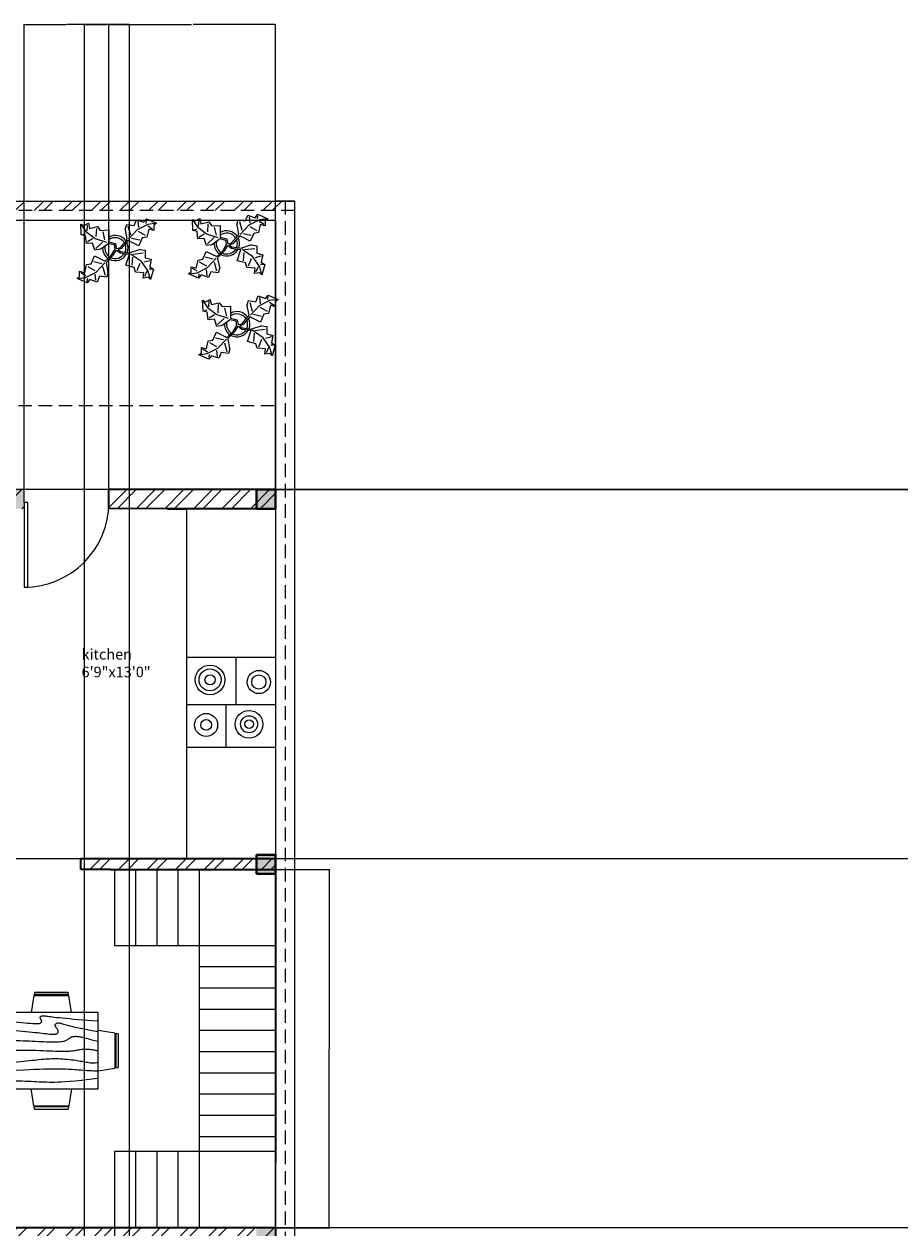
# Model space of a CAD drawing. Units: inches. Extents: x 19613 to 21413, y 12082 to 13202.
# Tile 6 of 9: x 20100 to 20513, y 12634 to 13202. Entities that reach past the tile are written whole.
import ezdxf

# ---------------------------------------------------------------- set-up
doc = ezdxf.new("R2010")
doc.units = ezdxf.units.IN
doc.linetypes.add('HIDDEN', pattern=[9.525, 6.35, -3.175])
for name, color, linetype, lineweight in [('A-ANNO-DIMS', 2, 'Continuous', 18), ('A-AREA-IDEN', 7, 'Continuous', 18), ('A-COLS', 7, 'Continuous', 40), ('A-COLS-PATT', 6, 'Continuous', 13), ('A-DOOR', 3, 'Continuous', 18), ('A-EQPM', 8, 'Continuous', 18), ('A-FLOR-CASE', 9, 'Continuous', 18), ('A-FLOR-HIDN', 8, 'HIDDEN', 13), ('A-FLOR-STRS', 7, 'Continuous', 18), ('A-FURN', 8, 'Continuous', 18), ('A-WALL', 7, 'Continuous', 35), ('A-WALL-PATT', 252, 'Continuous', 13), ('C-PROP', 7, 'Continuous', 25), ('C-PROP-HIDN', 8, 'HIDDEN', 13), ('L-PLNT', 116, 'Continuous', 18)]:
    doc.layers.add(name, color=color, linetype=linetype, lineweight=lineweight)
doc.styles.get("Standard").update_dxf_attribs({"font": 'arial.ttf'})
doc.dimstyles.get("Standard").update_dxf_attribs({"dimtxt": 0.18, "dimasz": 0.18, "dimexe": 0.18, "dimexo": 0.0625, "dimgap": 0.09, "dimtad": 0, "dimtih": 1, "dimtoh": 1, "dimdec": 4, "dimzin": 0, "dimdsep": 46, "dimtxsty": 'Standard', "dimcen": 0.09, "dimadec": 0, "dimazin": 0, "dimtfac": 1, "dimtdec": 4, "dimtofl": 0, "dimtmove": 0, "dimatfit": 3, "dimfxl": 1, "dimtolj": 1, "dimtzin": 0, "dimarcsym": 0})

# ---------------------------------------------------------------- blocks, each defined once
blk = doc.blocks.new('*U2')
for p, q in [((0, 0), (0, 6)), ((40, 0), (40, 6))]:
    blk.add_line(p, q)
blk.add_lwpolyline([(0, 0), (0, -40), (1.75, -40), (1.75, 0)], close=True)
blk.add_arc((0, 0), 40, 270, 0)
blk = doc.blocks.new('Dining Set - 36 x 72 in.')
for p, q in [((-22.2343, 26.00059), (-23.4847, 17.99762)), ((-22.2304, 26), (-5.7608, 26)), ((-22, 27.5), (-22.1562, 26.50042)), ((-5.8416, 26.5), (-22.1534, 26.5)), ((-22, 27.5), (-6, 27.5)), ((-5.8437, 26.49966), (-6, 27.5)), ((-4.5152, 17.99762), (-5.7655, 25.99926)), ((5.7657, 26.00059), (4.5153, 17.99762)), ((5.7696, 26), (22.2392, 26)), ((6, 27.5), (5.8438, 26.50042)), ((22.1584, 26.5), (5.8466, 26.5)), ((6, 27.5), (22, 27.5)), ((22.1563, 26.49966), (22, 27.5)), ((23.4848, 17.99762), (22.2345, 25.99926)), ((36, 18), (-36, 18)), ((-36, 18), (-36, -18)), ((36, -18), (36, 18)), ((-45.5, 8), (-44.5004, 8.15617)), ((-45.5, 8), (-45.5, -8)), ((-44.5, -8.15843), (-44.5, 8.15338)), ((-44.0006, 8.23428), (-35.9976, 9.48474)), ((-44, 8.23041), (-44, -8.23915)), ((44.0006, 8.23428), (35.9976, 9.48474)), ((44, 8.23041), (44, -8.23915)), ((44.5, -8.15843), (44.5, 8.15338)), ((45.5, 8), (44.5005, 8.15617)), ((45.5, 8), (45.5, -8)), ((-44.4997, -8.15631), (-45.5, -8)), ((-35.9976, -9.48476), (-43.9993, -8.2345)), ((35.9976, -9.48476), (43.9993, -8.2345)), ((44.4997, -8.15631), (45.5, -8)), ((-36, -18), (36, -18)), ((-22.2343, -26.0006), (-23.4847, -17.99762)), ((-4.5152, -17.99762), (-5.7655, -25.99928)), ((5.7657, -26.0006), (4.5153, -17.99762)), ((23.4848, -17.99762), (22.2345, -25.99928)), ((-22.2304, -26), (-5.7608, -26)), ((-22, -27.5), (-22.1562, -26.50044)), ((-5.8416, -26.5), (-22.1534, -26.5)), ((-22, -27.5), (-6, -27.5)), ((-5.8437, -26.49967), (-6, -27.5)), ((5.7696, -26), (22.2392, -26)), ((6, -27.5), (5.8438, -26.50044)), ((22.1584, -26.5), (5.8466, -26.5)), ((6, -27.5), (22, -27.5)), ((22.1563, -26.49967), (22, -27.5))]:
    blk.add_line(p, q)
for points in [[(-36, 15), (-31.1772, 14.97754), (-26.8079, 14.91406), (-22.8538, 14.81543), (-19.276, 14.6875), (-16.0362, 14.53613), (-13.0957, 14.36718), (-10.4159, 14.18652), (-7.9583, 14), (-5.6904, 13.81315), (-3.6035, 13.63021), (-1.6954, 13.45508), (0.0365, 13.29166), (1.5945, 13.14388), (2.9811, 13.01562), (4.1988, 12.9108), (5.25, 12.83333), (6.1393, 12.78613), (6.8802, 12.76823), (7.4883, 12.77767), (7.9792, 12.8125), (8.3685, 12.87077), (8.6719, 12.95052), (8.9049, 13.0498), (9.0833, 13.16666), (9.2205, 13.29899), (9.3216, 13.44401), (9.3895, 13.59879), (9.4271, 13.76041), (9.4373, 13.92594), (9.4232, 14.09245), (9.3875, 14.257), (9.3333, 14.41666), (9.2638, 14.56917), (9.1836, 14.71484), (9.0975, 14.85465), (9.0104, 14.98958), (8.9272, 15.1206), (8.8529, 15.2487), (8.7922, 15.37483), (8.75, 15.5), (8.7305, 15.62467), (8.7344, 15.74739), (8.7617, 15.86621), (8.8125, 15.97916), (8.8867, 16.08431), (8.9844, 16.17968), (9.1055, 16.26334), (9.25, 16.33333), (9.4189, 16.38802), (9.6172, 16.42708), (9.8506, 16.45052), (10.125, 16.45833), (10.4463, 16.45052), (10.8203, 16.42708), (11.2529, 16.38802), (11.75, 16.33333), (12.3184, 16.26318), (12.9694, 16.17838), (13.7151, 16.07991), (14.5677, 15.96875), (15.5395, 15.84586), (16.6426, 15.71224), (17.8893, 15.56884), (19.2917, 15.41666), (20.859, 15.25667), (22.5879, 15.08984), (24.4721, 14.91715), (26.5052, 14.73958), (28.6809, 14.5581), (30.9929, 14.3737), (33.4347, 14.18733), (36, 14)], [(-36, 10), (-28.9766, 10.14274), (-23.1725, 10.20442), (-18.4241, 10.19775), (-14.5677, 10.13541), (-11.4399, 10.03011), (-8.877, 9.89453), (-6.7154, 9.74137), (-4.7917, 9.58333), (-2.9698, 9.43082), (-1.2246, 9.28515), (0.4415, 9.14534), (2.026, 9.01041), (3.5266, 8.87939), (4.9408, 8.7513), (6.266, 8.62516), (7.5, 8.5), (8.6411, 8.37549), (9.6914, 8.2539), (10.6538, 8.13818), (11.5312, 8.03125), (12.3267, 7.93603), (13.043, 7.85547), (13.6831, 7.79248), (14.25, 7.75), (14.7471, 7.7303), (15.1797, 7.73307), (15.5537, 7.75732), (15.875, 7.80208), (16.1494, 7.86637), (16.3828, 7.94922), (16.5811, 8.04964), (16.75, 8.16666), (16.8944, 8.29915), (17.0143, 8.44531), (17.1089, 8.60319), (17.1771, 8.77083), (17.218, 8.94629), (17.2305, 9.1276), (17.2137, 9.31282), (17.1667, 9.5), (17.0895, 9.6875), (16.987, 9.875), (16.8649, 10.0625), (16.7292, 10.25), (16.5856, 10.4375), (16.4401, 10.625), (16.2985, 10.8125), (16.1667, 11), (16.05, 11.18733), (15.9518, 11.3737), (15.8752, 11.5581), (15.8229, 11.73958), (15.798, 11.91715), (15.8034, 12.08984), (15.842, 12.25667), (15.9167, 12.41666), (16.0295, 12.56836), (16.1784, 12.70833), (16.3605, 12.83268), (16.5729, 12.9375), (16.8127, 13.01888), (17.0768, 13.07291), (17.3625, 13.0957), (17.6667, 13.08333), (17.9894, 13.03312), (18.3418, 12.94726), (18.7382, 12.82918), (19.1927, 12.68229), (19.7195, 12.51001), (20.3327, 12.31575), (21.0465, 12.10294), (21.875, 11.875), (22.8357, 11.63354), (23.959, 11.37304), (25.2786, 11.08618), (26.8282, 10.76562), (28.6414, 10.40405), (30.752, 9.99414), (33.1936, 9.52856), (36, 9)], [(-36, 5.5), (-30.7157, 5.3348), (-26.069, 5.20963), (-21.9946, 5.11767), (-18.4271, 5.05208), (-15.3009, 5.00602), (-12.5508, 4.97265), (-10.1112, 4.94515), (-7.9167, 4.91666), (-5.909, 4.88167), (-4.0586, 4.83984), (-2.3429, 4.79215), (-0.7396, 4.73958), (0.7739, 4.6831), (2.22, 4.6237), (3.6213, 4.56233), (5, 4.5), (6.373, 4.43782), (7.7344, 4.3776), (9.0723, 4.32129), (10.375, 4.27083), (11.6309, 4.22819), (12.8281, 4.19531), (13.9551, 4.17415), (15, 4.16666), (15.954, 4.17448), (16.819, 4.19791), (17.6001, 4.23698), (18.3021, 4.29166), (18.9299, 4.36198), (19.4883, 4.44791), (19.9823, 4.54948), (20.4167, 4.66666), (20.7969, 4.79899), (21.1302, 4.94401), (21.4245, 5.09879), (21.6875, 5.26041), (21.9271, 5.42594), (22.1511, 5.59245), (22.3672, 5.757), (22.5834, 5.91666), (22.8065, 6.06868), (23.0404, 6.21093), (23.2879, 6.34147), (23.5521, 6.45833), (23.8358, 6.55957), (24.142, 6.64323), (24.4735, 6.70735), (24.8334, 6.75), (25.2235, 6.76969), (25.642, 6.76692), (26.0858, 6.74267), (26.5521, 6.69791), (27.0379, 6.63362), (27.5404, 6.55078), (28.0565, 6.45036), (28.5834, 6.33333), (29.1242, 6.19987), (29.7071, 6.04687), (30.3661, 5.87044), (31.1354, 5.66666), (32.0493, 5.43164), (33.142, 5.16146), (34.4475, 4.85221), (36, 4.5)], [(-36, -1), (-30.7915, -0.6591), (-26.0195, -0.38216), (-21.6519, -0.16284), (-17.6563, 0.00521), (-14.0005, 0.12833), (-10.6523, 0.21289), (-7.5796, 0.26522), (-4.75, 0.29166), (-2.134, 0.29793), (0.2878, 0.28711), (2.5317, 0.26163), (4.6146, 0.22396), (6.5529, 0.17651), (8.3633, 0.12174), (10.0623, 0.06209), (11.6667, 0), (13.1899, -0.06201), (14.6341, -0.1211), (15.9982, -0.17432), (17.2813, -0.21875), (18.4823, -0.25147), (19.6003, -0.26953), (20.6343, -0.27002), (21.5834, -0.25), (22.4481, -0.20768), (23.2357, -0.14584), (23.9549, -0.06836), (24.6146, 0.02083), (25.2235, 0.11784), (25.7904, 0.21875), (26.3241, 0.31966), (26.8334, 0.41666), (27.3265, 0.50618), (27.8099, 0.58593), (28.2894, 0.65397), (28.7709, 0.70833), (29.2601, 0.74707), (29.763, 0.76823), (30.2855, 0.76985), (30.8334, 0.75), (31.4088, 0.70784), (31.9994, 0.64713), (32.589, 0.57275), (33.1615, 0.48958), (33.7008, 0.4025), (34.1908, 0.3164), (34.6153, 0.23616), (34.9584, 0.16666), (35.2099, 0.11165), (35.3848, 0.07031), (35.504, 0.04069), (35.5886, 0.02083), (35.6594, 0.00879), (35.7377, 0.0026), (35.8442, 0.00032), (36, 0)], [(-36, -6.5), (-27.1843, -6.31267), (-20.084, -6.1263), (-14.469, -5.9419), (-10.1094, -5.76042), (-6.7752, -5.58285), (-4.2363, -5.41016), (-2.2629, -5.24333), (-0.625, -5.08334), (0.8708, -4.93099), (2.2715, -4.78646), (3.5872, -4.64974), (4.8281, -4.52084), (6.0046, -4.39974), (7.127, -4.28646), (8.2053, -4.18099), (9.25, -4.08334), (10.2705, -3.99382), (11.2734, -3.91407), (12.2647, -3.84603), (13.25, -3.79167), (14.2354, -3.75293), (15.2266, -3.73177), (16.2295, -3.73015), (17.25, -3.75), (18.2912, -3.79248), (19.3451, -3.85547), (20.4009, -3.93604), (21.4479, -4.03125), (22.4754, -4.13819), (23.4727, -4.25391), (24.4289, -4.37549), (25.3334, -4.5), (26.1785, -4.62492), (26.9694, -4.74935), (27.7145, -4.87281), (28.4219, -4.99479), (29.1, -5.11483), (29.7572, -5.23242), (30.4016, -5.34709), (31.0417, -5.45834), (31.6837, -5.56437), (32.3262, -5.65821), (32.9658, -5.73153), (33.599, -5.77604), (34.2224, -5.78345), (34.8327, -5.74545), (35.4264, -5.65373), (36, -5.5)], [(-36, -10), (-26.4022, -9.81299), (-18.4675, -9.62891), (-11.9839, -9.45069), (-6.7396, -9.28125), (-2.5226, -9.12354), (0.8789, -8.98047), (3.6769, -8.85498), (6.0833, -8.75), (8.2767, -8.66765), (10.3021, -8.60677), (12.1712, -8.56543), (13.8958, -8.54167), (15.4876, -8.53353), (16.9583, -8.53907), (18.3197, -8.55632), (19.5834, -8.58334), (20.7616, -8.61841), (21.8685, -8.66081), (22.9188, -8.71004), (23.9271, -8.76563), (24.9081, -8.82707), (25.8763, -8.89388), (26.8465, -8.96558), (27.8334, -9.04167), (28.8474, -9.12118), (29.8828, -9.20117), (30.93, -9.27824), (31.9792, -9.34896), (33.0205, -9.40991), (34.0443, -9.45768), (35.0407, -9.48885), (36, -9.5)], [(-36, -14.5), (-30.0881, -14.33513), (-25.0332, -14.21224), (-20.7312, -14.12647), (-17.0781, -14.07292), (-13.97, -14.04671), (-11.3027, -14.04297), (-8.9724, -14.05681), (-6.875, -14.08334), (-4.9224, -14.11833), (-3.0905, -14.16016), (-1.3709, -14.20785), (0.2448, -14.26042), (1.7647, -14.3169), (3.1973, -14.3763), (4.5507, -14.43767), (5.8333, -14.5), (7.0554, -14.5621), (8.235, -14.62175), (9.3922, -14.67652), (10.5469, -14.72396), (11.7192, -14.76164), (12.929, -14.78711), (14.1965, -14.79794), (15.5417, -14.79167), (16.9933, -14.76424), (18.6152, -14.70508), (20.4804, -14.60197), (22.6615, -14.44271), (25.2312, -14.21509), (28.2624, -13.9069), (31.8277, -13.50594), (36, -13)]]:
    blk.add_lwpolyline(points)
blk = doc.blocks.new('Plant - Rubber or Philodendron')
for p, q in [((-16.2005, 11.4774), (-13.9899, 8.1064)), ((-16.2005, 11.4774), (-14.8639, 10.7964)), ((-16.0159, 6.3329), (-16.2005, 11.4774)), ((-14.8639, 10.7964), (-12.6195, 11.8975)), ((-12.6195, 11.8975), (-12.1909, 9.4345)), ((8.8871, 10.7908), (9.9809, 13.4933)), ((9.9809, 13.4933), (13.3837, 12.301)), ((10.5828, 12.6946), (10.8893, 9.7953)), ((13.3837, 12.301), (14.68, 13.9039)), ((14.5816, 13.2037), (14.3848, 11.8033)), ((14.68, 13.9039), (19.3848, 11.8146)), ((19.3848, 11.8146), (15.3859, 11.3055)), ((19.3848, 11.8146), (18.1868, 10.9119)), ((-14.0069, 5.8704), (-16.0159, 6.3329)), ((-15.3434, 6.5514), (-13.9984, 6.9884)), ((-13.5868, 2.2894), (-14.0069, 5.8704)), ((-13.9899, 8.1064), (-9.5434, 4.7185)), ((-13.3174, 8.325), (-13.0735, 11.0065)), ((-12.1909, 9.4345), (-8.3829, 10.3)), ((-8.8369, 9.409), (-9.0894, 5.6095)), ((-8.3829, 10.3), (-7.0549, 8.501)), ((-7.0549, 8.501), (-3.0284, 8.6941)), ((-4.8529, 4.012), (-5.7184, 7.82)), ((-3.0284, 8.6941), (-3.0709, 3.1041)), ((4.6914, 8.8812), (5.3859, 11.2828)), ((4.6914, 8.8812), (5.5014, 4.4831)), ((5.3859, 11.2828), (8.8871, 10.7908)), ((5.9878, 10.4842), (7.1971, 6.3869)), ((10.3916, 8.7942), (6.2847, 4.4028)), ((15.3859, 11.3055), (10.3916, 8.7942)), ((14.2977, 6.1031), (10.9934, 7.9956)), ((15.7909, 9.1065), (14.8995, 5.3044)), ((15.2875, 10.6053), (17.5907, 9.2105)), ((18.1925, 8.4119), (15.7909, 9.1065)), ((18.1868, 10.9119), (18.1925, 8.4119)), ((-10.6784, 2.491), (-13.5868, 2.2894)), ((-13.1329, 3.1804), (-10.6614, 4.727)), ((-9.5858, -0.8715), (-10.6784, 2.491)), ((-9.5434, 4.7185), (-4.1917, 2.9888)), ((-9.1318, 0.0195), (-5.9793, 2.9025)), ((-7.1228, -0.443), (-3.5248, 2.2131)), ((-3.5248, 2.2131), (-3.3011, 2.4355)), ((-3.3011, 2.4355), (-0.5306, 1.7947)), ((-3.0709, 3.1041), (0.0797, 2.3163)), ((-0.5306, 1.7947), (-0.2255, -0.5527)), ((-0.5306, 1.7947), (-0.5306, 1.7947)), ((0.0797, 2.3163), (0.4866, -0.031)), ((0.4866, -0.031), (2.1141, 0.2298)), ((2.1141, 0.2298), (5.4346, 3.9146)), ((6.1032, 3.6844), (2.8262, -0.031)), ((5.4346, 3.9146), (5.5014, 4.4831)), ((11.1089, 1.1958), (6.1032, 3.6844)), ((7.7005, 4.8881), (11.5025, 3.9967)), ((12.7005, 4.8994), (11.1089, 1.1958)), ((14.8995, 5.3044), (12.7005, 4.8994)), ((-11.3237, -7.2629), (-9.7321, -3.5593)), ((-9.7321, -3.5593), (-4.7264, -6.0479)), ((-7.1228, -0.443), (-9.5858, -0.8715)), ((-2.019, -3.6148), (-4.7264, -6.0479)), ((-4.0579, -6.2781), (-0.9375, -3.1608)), ((-2.019, -3.6148), (-0.2255, -0.5527)), ((-0.9375, -3.1608), (0.5883, -0.8135)), ((0.5883, -0.8135), (2.2447, -2.0916)), ((2.8262, -0.031), (1.3003, -0.5527)), ((1.3003, -0.5527), (2.4193, -1.4655)), ((2.2447, -2.0916), (6.7108, -2.6626)), ((2.4193, -1.4655), (6.895, -2.1175)), ((4.943, -7.9659), (6.7108, -2.6626)), ((11.6605, -0.5413), (6.895, -2.1175)), ((12.3677, -6.1981), (7.219, -2.6772)), ((8.125, -4.0768), (7.7715, -7.9659)), ((8.3544, -2.7453), (13.1973, -2.1704)), ((11.6605, -0.5413), (14.1354, -0.8948)), ((14.1354, -0.8948), (14.1354, -4.4304)), ((14.1354, -4.4304), (16.9638, -5.1375)), ((16.9638, -5.1375), (16.2567, -8.673)), ((-16.8157, -10.7754), (-14.4141, -11.4699)), ((-16.8101, -13.2754), (-16.8157, -10.7754)), ((-14.4141, -11.4699), (-13.5228, -7.6679)), ((-14.0091, -13.669), (-9.0148, -11.1577)), ((-13.5228, -7.6679), (-11.3237, -7.2629)), ((-12.921, -8.4665), (-9.6166, -10.359)), ((-6.3237, -7.2516), (-10.1257, -6.3602)), ((-9.0148, -11.1577), (-4.9047, -6.8122)), ((-4.611, -12.8477), (-5.8203, -8.7504)), ((-4.1246, -6.8466), (-4.0579, -6.2781)), ((-3.3146, -11.2447), (-4.1246, -6.8466)), ((-3.3146, -11.2447), (-4.0092, -13.6463)), ((8.8321, -9.0266), (4.943, -7.9659)), ((9.5392, -11.1479), (8.8321, -9.0266)), ((13.4283, -11.5015), (9.5392, -11.1479)), ((10.2463, -10.4408), (11.6605, -6.9053)), ((15.5496, -10.7943), (12.3677, -6.1981)), ((16.2567, -5.8446), (13.4283, -6.5517)), ((14.8425, -10.7943), (13.7819, -13.2692)), ((16.6103, -14.6834), (15.5496, -10.7943)), ((17.3174, -9.7337), (15.9032, -9.7337)), ((16.2567, -8.673), (18.0245, -9.7337)), ((18.0245, -9.7337), (16.6103, -14.6834)), ((-18.008, -14.1781), (-16.8101, -13.2754)), ((-18.008, -14.1781), (-14.0091, -13.669)), ((-13.3032, -16.2674), (-18.008, -14.1781)), ((-13.9107, -12.9688), (-16.2139, -11.574)), ((-12.0069, -14.6645), (-13.3032, -16.2674)), ((-13.2048, -15.5672), (-13.008, -14.1668)), ((-8.6042, -15.8568), (-12.0069, -14.6645)), ((-9.206, -15.0581), (-9.5126, -12.1588)), ((-7.5103, -13.1543), (-8.6042, -15.8568)), ((-4.0092, -13.6463), (-7.5103, -13.1543)), ((13.0748, -13.9763), (13.4283, -11.5015)), ((15.5496, -13.6228), (13.0748, -13.9763)), ((16.6103, -14.6834), (15.5496, -13.6228))]:
    blk.add_line(p, q)
for centre, radius, start, end in [((0, 0), 6.1275, 34.37569, 120.1028), ((0.0308, 0.1664), 6, 178.6147, 235.1169), ((0.0308, 0.1664), 5, 168.1647, 238.6725), ((-0.0601, -0.2075), 5.2461, 33.82192, 124.9414), ((-0.2664, 0.1682), 5.2775, 338.4094, 20.03007), ((-0.098, 0.1364), 6.1288, 341.2017, 26.09184), ((-0.0234, 0.3825), 6.1492, 242.5812, 331.2714), ((-0.1102, 0.4886), 5.2883, 247.3711, 327.472)]:
    blk.add_arc(centre, radius, start, end)
blk = doc.blocks.new('COL-9x9')
for p, q in [((0, 9), (9, 9)), ((0, 0), (0, 9)), ((9, 9), (9, 0)), ((9, 0), (0, 0))]:
    blk.add_line(p, q)
blk = doc.blocks.new('RANGE-4-BURNER')
for p, q in [((42, 42.44), (0, 42.44)), ((23.29, 42.44), (23.29, 20.04)), ((42, 20.04), (0, 20.04)), ((18.54, 20.04), (18.54, 0)), ((42, 0), (0, 0))]:
    blk.add_line(p, q)
for centre, radius in [((11.11, 31.86), 6.98), ((11.11, 31.86), 5.19), ((11.11, 31.86), 2.41), ((34.12, 30.84), 5.47), ((34.12, 30.84), 3.36), ((34.12, 30.84), 3.36), ((34.12, 30.84), 3.36), ((29.52, 10.94), 6.53), ((29.52, 10.94), 6.53), ((29.52, 10.94), 6.53), ((9.27, 10.62), 5.42), ((9.27, 10.62), 2.53), ((29.52, 10.94), 4.03), ((29.52, 10.94), 2.04)]:
    blk.add_circle(centre, radius)
blk = doc.blocks.new('STAIR-RETURN-FLIGHT')
for p, q in [((0, 169), (0, 133)), ((10, 169), (10, 133)), ((20, 169), (20, 133)), ((30, 169), (30, 133)), ((76, 169), (40, 169)), ((76, 169), (40, 169)), ((40, 169), (40, 0)), ((76, 169), (76, 133)), ((76, 169), (76, 133)), ((76, 133), (0, 133)), ((76, 123), (40, 123)), ((76, 113), (40, 113)), ((76, 103), (40, 103)), ((76, 93), (40, 93)), ((76, 83), (40, 83)), ((76, 73), (40, 73)), ((76, 63), (40, 63)), ((76, 31), (76, 67)), ((76, 53), (40, 53)), ((76, 43), (40, 43)), ((76, 36), (0, 36)), ((0, 36), (0, 0)), ((10, 36), (10, 0)), ((20, 36), (20, 0)), ((30, 36), (30, 0)), ((76, 0), (76, 36))]:
    blk.add_line(p, q)
blk = doc.blocks.new('*D77')
at = {"layer": 'A-ANNO-DIMS', "color": 0, "lineweight": -2, "transparency": 16777216}
for p, q in [((20218.76, 12803.28), (20244.22, 12803.28)), ((20244.04, 12803.1), (20244.04, 12718.96)), ((20244.04, 12634.46), (20244.04, 12718.6)), ((20218.76, 12634.28), (20244.22, 12634.28))]:
    blk.add_line(p, q, dxfattribs=at)
at = {"layer": 'A-ANNO-DIMS', "color": 0, "transparency": 16777216}
for points in [[(20244.01, 12803.1), (20244.07, 12803.1), (20244.04, 12803.28)], [(20244.01, 12634.46), (20244.07, 12634.46), (20244.04, 12634.28)]]:
    blk.add_solid(points, dxfattribs=at)
at = {"layer": 'Defpoints', "color": 0, "transparency": 16777216}
for p in [(20218.69, 12803.28), (20244.04, 12803.28), (20218.69, 12634.28)]:
    blk.add_point(p, dxfattribs=at)
at = {"layer": 'A-ANNO-DIMS', "color": 0, "transparency": 16777216, "insert": (20244.04, 12718.78), "char_height": 0.18, "attachment_point": 5}
blk.add_mtext('\\A1;STAIR 169 TYP.', dxfattribs=at)
blk = doc.blocks.new('*D78')
at = {"layer": 'A-ANNO-DIMS', "color": 0, "lineweight": -2, "transparency": 16777216}
for p, q in [((20142.69, 12634.22), (20142.69, 12608.75)), ((20218.69, 12634.22), (20218.69, 12608.75)), ((20142.87, 12608.93), (20180.17, 12608.93)), ((20218.51, 12608.93), (20181.22, 12608.93))]:
    blk.add_line(p, q, dxfattribs=at)
at = {"layer": 'A-ANNO-DIMS', "color": 0, "transparency": 16777216}
for points in [[(20142.87, 12608.96), (20142.87, 12608.9), (20142.69, 12608.93)], [(20218.51, 12608.96), (20218.51, 12608.9), (20218.69, 12608.93)]]:
    blk.add_solid(points, dxfattribs=at)
at = {"layer": 'Defpoints', "color": 0, "transparency": 16777216}
for p in [(20142.69, 12634.28), (20218.69, 12634.28), (20218.69, 12608.93)]:
    blk.add_point(p, dxfattribs=at)
at = {"layer": 'A-ANNO-DIMS', "color": 0, "transparency": 16777216, "insert": (20180.69, 12608.93), "char_height": 0.18, "attachment_point": 5}
blk.add_mtext('\\A1;76 TYP.', dxfattribs=at)
blk = doc.blocks.new('*D87')
at = {"layer": 'A-ANNO-DIMS', "color": 0, "lineweight": -2, "transparency": 16777216}
for p, q in [((20218.76, 12982.28), (21412.86, 12982.28)), ((21412.68, 12982.1), (21412.68, 12697.46)), ((21412.68, 12412.46), (21412.68, 12697.1)), ((20218.76, 12412.28), (21412.86, 12412.28))]:
    blk.add_line(p, q, dxfattribs=at)
at = {"layer": 'A-ANNO-DIMS', "color": 0, "transparency": 16777216}
for points in [[(21412.65, 12982.1), (21412.71, 12982.1), (21412.68, 12982.28)], [(21412.65, 12412.46), (21412.71, 12412.46), (21412.68, 12412.28)]]:
    blk.add_solid(points, dxfattribs=at)
at = {"layer": 'Defpoints', "color": 0, "transparency": 16777216}
for p in [(20218.69, 12982.28), (21412.68, 12982.28), (20218.69, 12412.28)]:
    blk.add_point(p, dxfattribs=at)
at = {"layer": 'A-ANNO-DIMS', "color": 0, "transparency": 16777216, "insert": (21412.68, 12697.28), "char_height": 0.18, "attachment_point": 5}
blk.add_mtext('\\A1;570', dxfattribs=at)
blk = doc.blocks.new('*D89')
at = {"layer": 'A-ANNO-DIMS', "color": 0, "lineweight": -2, "transparency": 16777216}
for p, q in [((20807.37, 12808.28), (19613.26, 12808.28)), ((19613.44, 12808.1), (19613.44, 12721.46)), ((19613.44, 12634.46), (19613.44, 12721.1)), ((20807.37, 12634.28), (19613.26, 12634.28))]:
    blk.add_line(p, q, dxfattribs=at)
at = {"layer": 'A-ANNO-DIMS', "color": 0, "transparency": 16777216}
for points in [[(19613.41, 12808.1), (19613.47, 12808.1), (19613.44, 12808.28)], [(19613.41, 12634.46), (19613.47, 12634.46), (19613.44, 12634.28)]]:
    blk.add_solid(points, dxfattribs=at)
at = {"layer": 'Defpoints', "color": 0, "transparency": 16777216}
for p in [(19613.44, 12808.28), (20807.43, 12808.28), (20807.43, 12634.28)]:
    blk.add_point(p, dxfattribs=at)
at = {"layer": 'A-ANNO-DIMS', "color": 0, "transparency": 16777216, "insert": (19613.44, 12721.28), "char_height": 0.18, "attachment_point": 5}
blk.add_mtext('\\A1;174', dxfattribs=at)
blk = doc.blocks.new('*D90')
at = {"layer": 'A-ANNO-DIMS', "color": 0, "lineweight": -2, "transparency": 16777216}
for p, q in [((20807.37, 12982.28), (19613.26, 12982.28)), ((19613.44, 12982.1), (19613.44, 12895.46)), ((19613.44, 12808.46), (19613.44, 12895.1)), ((20807.37, 12808.28), (19613.26, 12808.28))]:
    blk.add_line(p, q, dxfattribs=at)
at = {"layer": 'A-ANNO-DIMS', "color": 0, "transparency": 16777216}
for points in [[(19613.41, 12982.1), (19613.47, 12982.1), (19613.44, 12982.28)], [(19613.41, 12808.46), (19613.47, 12808.46), (19613.44, 12808.28)]]:
    blk.add_solid(points, dxfattribs=at)
at = {"layer": 'Defpoints', "color": 0, "transparency": 16777216}
for p in [(19613.44, 12982.28), (20807.43, 12982.28), (20807.43, 12808.28)]:
    blk.add_point(p, dxfattribs=at)
at = {"layer": 'A-ANNO-DIMS', "color": 0, "transparency": 16777216, "insert": (19613.44, 12895.28), "char_height": 0.18, "attachment_point": 5}
blk.add_mtext('\\A1;174', dxfattribs=at)
blk = doc.blocks.new('*D94')
at = {"layer": 'A-ANNO-DIMS', "color": 0, "lineweight": -2, "transparency": 16777216}
for p, q in [((20100.12, 12982.34), (20100.12, 13201.71)), ((20100.3, 13201.53), (20119.9, 13201.53)), ((20139.94, 13201.53), (20120.34, 13201.53)), ((20140.12, 12982.34), (20140.12, 13201.71))]:
    blk.add_line(p, q, dxfattribs=at)
at = {"layer": 'A-ANNO-DIMS', "color": 0, "transparency": 16777216}
for points in [[(20100.3, 13201.56), (20100.3, 13201.5), (20100.12, 13201.53)], [(20139.94, 13201.56), (20139.94, 13201.5), (20140.12, 13201.53)]]:
    blk.add_solid(points, dxfattribs=at)
at = {"layer": 'Defpoints', "color": 0, "transparency": 16777216}
for p in [(20140.12, 13201.53), (20100.12, 12982.28), (20140.12, 12982.28)]:
    blk.add_point(p, dxfattribs=at)
at = {"layer": 'A-ANNO-DIMS', "color": 0, "transparency": 16777216, "insert": (20120.12, 13201.53), "char_height": 0.18, "attachment_point": 5}
blk.add_mtext('\\A1;40', dxfattribs=at)
blk = doc.blocks.new('*D95')
at = {"layer": 'A-ANNO-DIMS', "color": 0, "lineweight": -2, "transparency": 16777216}
for p, q in [((20140.12, 12982.34), (20140.12, 13201.71)), ((20140.3, 13201.53), (20179.01, 13201.53)), ((20218.51, 13201.53), (20179.8, 13201.53)), ((20218.69, 12982.34), (20218.69, 13201.71))]:
    blk.add_line(p, q, dxfattribs=at)
at = {"layer": 'A-ANNO-DIMS', "color": 0, "transparency": 16777216}
for points in [[(20140.3, 13201.56), (20140.3, 13201.5), (20140.12, 13201.53)], [(20218.51, 13201.56), (20218.51, 13201.5), (20218.69, 13201.53)]]:
    blk.add_solid(points, dxfattribs=at)
at = {"layer": 'Defpoints', "color": 0, "transparency": 16777216}
for p in [(20218.69, 13201.53), (20140.12, 12982.28), (20218.69, 12982.28)]:
    blk.add_point(p, dxfattribs=at)
at = {"layer": 'A-ANNO-DIMS', "color": 0, "transparency": 16777216, "insert": (20179.41, 13201.53), "char_height": 0.18, "attachment_point": 5}
blk.add_mtext('\\A1;78.57', dxfattribs=at)
blk = doc.blocks.new('*D107')
at = {"layer": 'A-ANNO-DIMS', "color": 0, "lineweight": -2, "transparency": 16777216}
for p, q in [((20128.69, 12412.34), (20128.69, 13201.71)), ((20128.87, 13201.53), (20138.81, 13201.53)), ((20149.67, 13201.53), (20139.74, 13201.53)), ((20149.85, 12412.34), (20149.85, 13201.71))]:
    blk.add_line(p, q, dxfattribs=at)
at = {"layer": 'A-ANNO-DIMS', "color": 0, "transparency": 16777216}
for points in [[(20128.87, 13201.56), (20128.87, 13201.5), (20128.69, 13201.53)], [(20149.67, 13201.56), (20149.67, 13201.5), (20149.85, 13201.53)]]:
    blk.add_solid(points, dxfattribs=at)
at = {"layer": 'Defpoints', "color": 0, "transparency": 16777216}
for p in [(20149.85, 13201.53), (20128.69, 12412.28), (20149.85, 12412.28)]:
    blk.add_point(p, dxfattribs=at)
at = {"layer": 'A-ANNO-DIMS', "color": 0, "transparency": 16777216, "insert": (20139.27, 13201.53), "char_height": 0.18, "attachment_point": 5}
blk.add_mtext('\\A1;21.154', dxfattribs=at)

msp = doc.modelspace()

# ---------------------------------------------------------------- hatches: boundary and pattern name
at = {"layer": 'A-COLS-PATT'}
h = msp.add_hatch(color=256, dxfattribs=at)
h.dxf.hatch_style = 1
h.paths.add_polyline_path([(19701.1937, 13118.279), (19696.6937, 13118.279), (19696.6937, 13113.779), (19701.1937, 13113.779)])
h.paths.add_polyline_path([(19714.6694, 12982.279), (19705.6937, 12982.279), (19705.6937, 12973.279), (19714.6694, 12973.279)])
h.paths.add_polyline_path([(19827.1183, 12982.279), (19818.1183, 12982.279), (19818.1183, 12973.279), (19827.1183, 12973.279)])
h.paths.add_polyline_path([(19982.6937, 12982.279), (19973.6937, 12982.279), (19973.6937, 12973.279), (19982.6937, 12973.279)])
h.paths.add_polyline_path([(19982.6937, 12817.279), (19973.6937, 12817.279), (19973.6937, 12808.279), (19982.6937, 12808.279)])
h.paths.add_polyline_path([(19795.361, 12817.279), (19786.361, 12817.279), (19786.361, 12808.279), (19795.361, 12808.279)])
h.paths.add_polyline_path([(19705.6937, 12817.279), (19702.0819, 12817.279), (19702.0819, 12808.279), (19705.6937, 12808.279)])
h.paths.add_polyline_path([(19711.0819, 12817.279), (19705.6937, 12817.279), (19705.6937, 12808.279), (19711.0819, 12808.279)])
h.paths.add_polyline_path([(19714.6136, 12634.279), (19705.6937, 12634.279), (19705.6937, 12625.279), (19714.6136, 12625.279)])
h.paths.add_polyline_path([(19705.6937, 12485.8897), (19701.1937, 12485.8897), (19701.1937, 12476.8897), (19705.6937, 12476.8897)])
h.paths.add_polyline_path([(19709.3479, 12485.8897), (19705.6937, 12485.8897), (19705.6937, 12476.8897), (19709.3479, 12476.8897)])
h.paths.add_polyline_path([(19701.1937, 12485.8897), (19700.3479, 12485.8897), (19700.3479, 12476.8897), (19701.1937, 12476.8897)])
h.paths.add_polyline_path([(20218.6937, 12421.279), (20209.6937, 12421.279), (20209.6937, 12412.279), (20218.6937, 12412.279)])
h.paths.add_polyline_path([(20218.6937, 12634.279), (20209.6937, 12634.279), (20209.6937, 12625.279), (20218.6937, 12625.279)])
h.paths.add_polyline_path([(20218.6937, 12808.279), (20209.6937, 12808.279), (20209.6937, 12803.279), (20218.6937, 12803.279)])
h.paths.add_polyline_path([(20218.6937, 12810.1878), (20209.6937, 12810.1878), (20209.6937, 12808.279), (20218.6937, 12808.279)])
h.paths.add_polyline_path([(20218.6937, 12803.279), (20209.6937, 12803.279), (20209.6937, 12801.1878), (20218.6937, 12801.1878)])
h.paths.add_polyline_path([(20218.6937, 12982.279), (20209.6937, 12982.279), (20209.6937, 12973.279), (20218.6937, 12973.279)])
h.paths.add_polyline_path([(20100.1214, 12982.279), (20080.8386, 12982.279), (20080.8386, 12973.279), (20091.6937, 12973.279), (20100.1214, 12973.279), (20100.1214, 12976.279)])
h.paths.add_polyline_path([(19851.5503, 12631.279), (19851.5503, 12634.279), (19828.8814, 12634.279), (19828.8814, 12625.279), (19851.5503, 12625.279)])
at = {"layer": 'A-WALL-PATT'}
h = msp.add_hatch(dxfattribs=at)
h.set_pattern_fill('ANSI32', color=256)
h.paths.add_polyline_path([(20223.1937, 13118.279), (20218.6937, 13118.279), (19701.1937, 13118.279), (19701.1937, 13113.779), (20223.1937, 13113.779)])
h.paths.add_polyline_path([(19849.7315, 12982.279), (19799.9854, 12982.279), (19799.9854, 12973.279), (19849.7315, 12973.279)])
h.paths.add_polyline_path([(19755.5378, 12982.279), (19705.6937, 12982.279), (19705.6937, 12973.279), (19755.5378, 12973.279)])
h.paths.add_polyline_path([(20000.1054, 12982.279), (19950.0534, 12982.279), (19950.0534, 12974.1171), (19950.0534, 12973.279), (20000.1054, 12973.279)])
h.paths.add_polyline_path([(20049.4797, 12982.279), (20030.7476, 12982.279), (20030.7476, 12973.279), (20049.4797, 12973.279)])
h.paths.add_polyline_path([(20100.1214, 12982.279), (20080.8386, 12982.279), (20080.8386, 12973.279), (20100.1214, 12973.279), (20100.1214, 12976.279)])
h.paths.add_polyline_path([(20218.6937, 12982.279), (20167.6937, 12982.279), (20140.1214, 12982.279), (20140.1214, 12976.279, -0.01769781), (20140.0212, 12973.45), (20167.6937, 12973.279), (20176.6937, 12973.279), (20218.6937, 12973.279)])
h.paths.add_polyline_path([(19851.5503, 12814.279), (19851.5503, 12817.279), (19793.6937, 12817.279), (19789.6937, 12817.279), (19705.6937, 12817.279), (19705.6937, 12808.279), (19851.5503, 12808.279)])
h.paths.add_polyline_path([(19982.6937, 12973.279), (19973.6937, 12973.279), (19973.6937, 12817.279), (19887.5503, 12817.279), (19887.5503, 12808.279), (19973.6937, 12808.279), (19982.6937, 12808.279)])
h.paths.add_polyline_path([(20058.6937, 12850.5529), (19982.6937, 12850.5529), (19982.6937, 12846.5529), (20058.6937, 12846.5529)])
h.paths.add_polyline_path([(20095.6937, 12973.279), (20091.6937, 12973.279), (20091.6937, 12850.5529), (20087.6937, 12850.5529), (20087.6937, 12846.5529), (20095.6937, 12846.5529)])
h.paths.add_polyline_path([(20218.6937, 12808.279), (20140.8605, 12808.279), (20126.9413, 12808.279), (20126.9413, 12803.279), (20140.8605, 12803.279), (20218.6937, 12803.279)])
h.paths.add_polyline_path([(19738.3931, 12634.279), (19705.6937, 12634.279), (19705.6937, 12625.279), (19738.3931, 12625.279)])
h.paths.add_polyline_path([(19912.6937, 12634.279), (19903.6937, 12634.279), (19891.5503, 12634.279), (19891.5503, 12625.279), (19903.6937, 12625.279), (19903.6937, 12445.279), (19975.6937, 12445.279), (20128.6937, 12445.279), (20128.6937, 12412.279), (20149.8479, 12412.279), (20149.8479, 12421.279), (20137.6937, 12421.279), (20137.6937, 12454.279), (20137.6937, 12580.2801), (20133.6937, 12580.2801), (20133.6937, 12454.279), (19984.6937, 12454.279), (19984.6937, 12625.279), (19993.6937, 12625.279), (19993.6937, 12634.279), (19984.6937, 12634.279), (19975.6937, 12634.279), (19975.6937, 12454.279), (19912.6937, 12454.279)])
h.paths.add_polyline_path([(20218.6937, 12634.279), (20137.6937, 12634.279), (20029.6937, 12634.279), (20029.6937, 12625.279), (20137.6937, 12625.279), (20218.6937, 12625.279)])
h.paths.add_polyline_path([(21014.4339, 12634.279), (21005.4339, 12634.279), (20993.2905, 12634.279), (20993.2905, 12625.279), (21005.4339, 12625.279), (21005.4339, 12445.279), (21077.4339, 12445.279), (21230.4339, 12445.279), (21230.4339, 12412.279), (21251.5881, 12412.279), (21251.5881, 12421.279), (21239.4339, 12421.279), (21239.4339, 12454.279), (21239.4339, 12580.2801), (21235.4339, 12580.2801), (21235.4339, 12454.279), (21086.4339, 12454.279), (21086.4339, 12625.279), (21095.4339, 12625.279), (21095.4339, 12634.279), (21086.4339, 12634.279), (21077.4339, 12634.279), (21077.4339, 12454.279), (21014.4339, 12454.279)])
h.paths.add_polyline_path([(20840.1333, 12634.279), (20807.4339, 12634.279), (20807.4339, 12625.279), (20840.1333, 12625.279)])
h.paths.add_polyline_path([(20953.2905, 12631.279), (20953.2905, 12634.279), (20930.6216, 12634.279), (20930.6216, 12625.279), (20953.2905, 12625.279)])
h.paths.add_polyline_path([(21320.4339, 12634.279), (21239.4339, 12634.279), (21131.4339, 12634.279), (21131.4339, 12625.279), (21239.4339, 12625.279), (21320.4339, 12625.279)])
h.paths.add_polyline_path([(21084.4339, 12973.279), (21075.4339, 12973.279), (21075.4339, 12817.279), (20989.2905, 12817.279), (20989.2905, 12808.279), (21075.4339, 12808.279), (21084.4339, 12808.279)])
h.paths.add_polyline_path([(21142.1261, 12863.2893), (21084.4339, 12863.2893), (21084.4339, 12846.5529), (21142.1261, 12846.5529)])
h.paths.add_polyline_path([(21320.4339, 12808.279), (21242.6007, 12808.279), (21228.6815, 12808.279), (21228.6815, 12803.279), (21242.6007, 12803.279), (21320.4339, 12803.279)])
h.paths.add_polyline_path([(20857.278, 12982.279), (20807.4339, 12982.279), (20807.4339, 12973.279), (20857.278, 12973.279)])
h.paths.add_polyline_path([(20951.4717, 12982.279), (20901.7255, 12982.279), (20901.7255, 12973.279), (20951.4717, 12973.279)])
h.paths.add_polyline_path([(21101.8455, 12982.279), (21051.7936, 12982.279), (21051.7936, 12974.1171), (21051.7936, 12973.279), (21101.8455, 12973.279)])
h.paths.add_polyline_path([(21151.2199, 12982.279), (21132.4878, 12982.279), (21132.4878, 12973.279), (21151.2199, 12973.279)])
h.paths.add_polyline_path([(21201.8616, 12982.279), (21182.5788, 12982.279), (21182.5788, 12973.279), (21193.4339, 12973.279), (21201.8616, 12973.279), (21201.8616, 12976.279)])
h.paths.add_polyline_path([(21320.4339, 12982.279), (21269.4339, 12982.279), (21241.8616, 12982.279), (21241.8616, 12976.279, -0.01769781), (21241.7614, 12973.45), (21269.4339, 12973.279), (21278.4339, 12973.279), (21320.4339, 12973.279)])
h.paths.add_polyline_path([(20953.2905, 12817.279), (20895.4339, 12817.279), (20891.4339, 12817.279), (20807.4339, 12817.279), (20807.4339, 12808.279), (20953.2905, 12808.279)])
h.paths.add_polyline_path([(21197.4339, 12973.279), (21193.4339, 12973.279), (21193.4339, 12850.5529), (21197.4339, 12850.5529)])
h.paths.add_polyline_path([(21320.4339, 12550.279), (21272.5278, 12550.279), (21272.5278, 12546.279), (21320.4339, 12546.279)])
h.paths.add_polyline_path([(21320.4339, 12421.279), (21283.2222, 12421.279), (21283.2222, 12412.279), (21320.4339, 12412.279)])

# ---------------------------------------------------------------- linework, layer by layer
at = {"layer": 'A-FLOR-CASE'}
for p, q in [((20176.6937, 12973.279), (20176.6937, 12808.279)), ((20176.6937, 12808.279), (20218.6937, 12808.279))]:
    msp.add_line(p, q, dxfattribs=at)
at = {"layer": 'A-FLOR-HIDN'}
msp.add_line((20030.7476, 13021.8552), (20218.6937, 13021.8552), dxfattribs=at)
at = {"layer": 'A-WALL'}
for p, q in [((20140.0212, 12973.45), (20140.1214, 12982.279)), ((20167.6937, 12982.279), (20140.1214, 12982.279)), ((20218.6937, 12982.279), (20167.6937, 12982.279)), ((20167.6937, 12973.279), (20140.0212, 12973.45)), ((20218.6937, 12973.279), (20167.6937, 12973.279)), ((20176.6937, 12973.279), (20167.6937, 12973.279)), ((20167.6937, 12973.279), (20176.6937, 12973.279)), ((20140.8605, 12808.279), (20126.9413, 12808.279)), ((20126.9413, 12803.279), (20126.9413, 12808.279)), ((20218.6937, 12808.279), (20140.8605, 12808.279)), ((20140.8605, 12803.279), (20126.9413, 12803.279)), ((20140.8605, 12803.279), (20218.6937, 12803.279)), ((20218.6937, 12803.279), (20218.6937, 12665.279)), ((20137.6937, 12634.279), (20029.6937, 12634.279)), ((20218.6937, 12634.279), (20137.6937, 12634.279)), ((20218.6937, 12634.279), (20218.6937, 12550.279))]:
    msp.add_line(p, q, dxfattribs=at)
at = {"layer": 'C-PROP'}
for p, q in [((19696.6937, 13118.279), (20227.6937, 13118.279)), ((20227.6937, 13118.279), (20218.6937, 13118.279)), ((20227.6937, 13118.279), (20223.1937, 13118.279)), ((20227.6937, 13118.279), (20227.6937, 12175.279)), ((20227.6937, 13118.279), (20227.6937, 13113.779)), ((20227.6937, 13113.779), (20227.6937, 12986.779)), ((19705.6937, 13109.279), (20218.6937, 13109.279)), ((20218.6937, 13109.279), (20218.6937, 12184.279)), ((20218.6937, 13109.279), (20218.6937, 12982.279))]:
    msp.add_line(p, q, dxfattribs=at)
at = {"layer": 'C-PROP-HIDN'}
for p, q in [((20227.6937, 13113.779), (19696.6937, 13113.779)), ((20223.1937, 13118.279), (20223.1937, 12175.279))]:
    msp.add_line(p, q, dxfattribs=at)

# ---------------------------------------------------------------- block references
at = {"layer": 'A-COLS', "rotation": 180}
for p in [(20218.6941, 12982.279), (20218.6941, 12810.1878)]:
    msp.add_blockref('COL-9x9', p, dxfattribs=at)
at = {"layer": 'A-DOOR'}
msp.add_blockref('*U2', (20100.1214, 12976.279), dxfattribs=at)
at = {"layer": 'A-EQPM'}
msp.add_blockref('RANGE-4-BURNER', (20176.694, 12860.744), dxfattribs=at)
at = {"layer": 'A-FLOR-STRS'}
msp.add_blockref('STAIR-RETURN-FLIGHT', (20142.694, 12634.279), dxfattribs=at)
at = {"layer": 'A-FURN'}
msp.add_blockref('Dining Set - 36 x 72 in.', (20098.9872, 12717.8276), dxfattribs=at)
at = {"layer": 'L-PLNT'}
for p in [(20143.1221, 13095.9866), (20195.6703, 13098.1393), (20200.5181, 13060.0608)]:
    msp.add_blockref('Plant - Rubber or Philodendron', p, dxfattribs=at)

# ---------------------------------------------------------------- texts
at = {"layer": 'A-AREA-IDEN', "insert": (20127.2168, 12907.1578), "char_height": 5, "attachment_point": 1}
msp.add_mtext_dynamic_manual_height_columns('kitchen\\P6\'9"x13\'0"', width=19.652904, gutter_width=12.5, heights=[0], dxfattribs=at)

# ---------------------------------------------------------------- dimensions: what is measured, and where the dimension line sits
at = {"layer": 'A-ANNO-DIMS'}
for base, p1, p2, override, picture, middle in [((20140.1214, 13201.529), (20100.1214, 12982.279), (20140.1214, 12982.279), {"dimdec": 0, "dimlfac": 1, "dimrnd": 0, "dimzin": 0, "dimdsep": 46, "dimlunit": 2}, '*D94', (20120.1214, 13201.529)), ((20149.8479, 13201.529), (20128.6937, 12412.279), (20149.8479, 12412.279), {"dimdec": 3, "dimlfac": 1, "dimrnd": 0, "dimzin": 0, "dimdsep": 46, "dimlunit": 2}, '*D107', (20139.2708, 13201.529)), ((20218.6937, 13201.529), (20140.1214, 12982.279), (20218.6937, 12982.279), {"dimdec": 2, "dimlfac": 1, "dimrnd": 0, "dimzin": 0, "dimdsep": 46, "dimlunit": 2}, '*D95', (20179.4075, 13201.529))]:
    dim = msp.add_linear_dim(base=base, p1=p1, p2=p2, dimstyle='Standard', override=override, dxfattribs=at)
    dim.commit()
    dim.dimension.update_dxf_attribs({"geometry": picture, "text_midpoint": middle})
for base, p1, p2, picture, middle in [((19613.4437, 12982.279), (20807.4339, 12808.279), (20807.4328, 12982.279), '*D90', (19613.4437, 12895.279)), ((21412.6839, 12982.279), (20218.6937, 12412.279), (20218.6937, 12982.279), '*D87', (21412.6839, 12697.279)), ((19613.4437, 12808.279), (20807.4339, 12634.279), (20807.4339, 12808.279), '*D89', (19613.4437, 12721.279))]:
    dim = msp.add_linear_dim(base=base, p1=p1, p2=p2, angle=90, dimstyle='Standard', override={"dimdec": 0, "dimlfac": 1, "dimrnd": 0, "dimzin": 0, "dimdsep": 46, "dimlunit": 2}, dxfattribs=at)
    dim.commit()
    dim.dimension.update_dxf_attribs({"geometry": picture, "text_midpoint": middle})
dim = msp.add_linear_dim(base=(20244.0437, 12803.279), p1=(20218.6937, 12634.279), p2=(20218.6937, 12803.279), angle=90, text='STAIR <> TYP.', dimstyle='Standard', override={"dimdec": 0, "dimlfac": 1, "dimrnd": 0, "dimzin": 0, "dimdsep": 46, "dimlunit": 2}, dxfattribs=at)
dim.commit()
dim.dimension.update_dxf_attribs({"geometry": '*D77', "text_midpoint": (20244.0437, 12718.779)})
dim = msp.add_linear_dim(base=(20218.6937, 12608.929), p1=(20142.6937, 12634.279), p2=(20218.6937, 12634.279), text='<> TYP.', dimstyle='Standard', override={"dimdec": 0, "dimlfac": 1, "dimrnd": 0, "dimzin": 0, "dimdsep": 46, "dimlunit": 2}, dxfattribs=at)
dim.commit()
dim.dimension.update_dxf_attribs({"geometry": '*D78', "text_midpoint": (20180.6937, 12608.929)})

doc.saveas('drawing.dxf')
